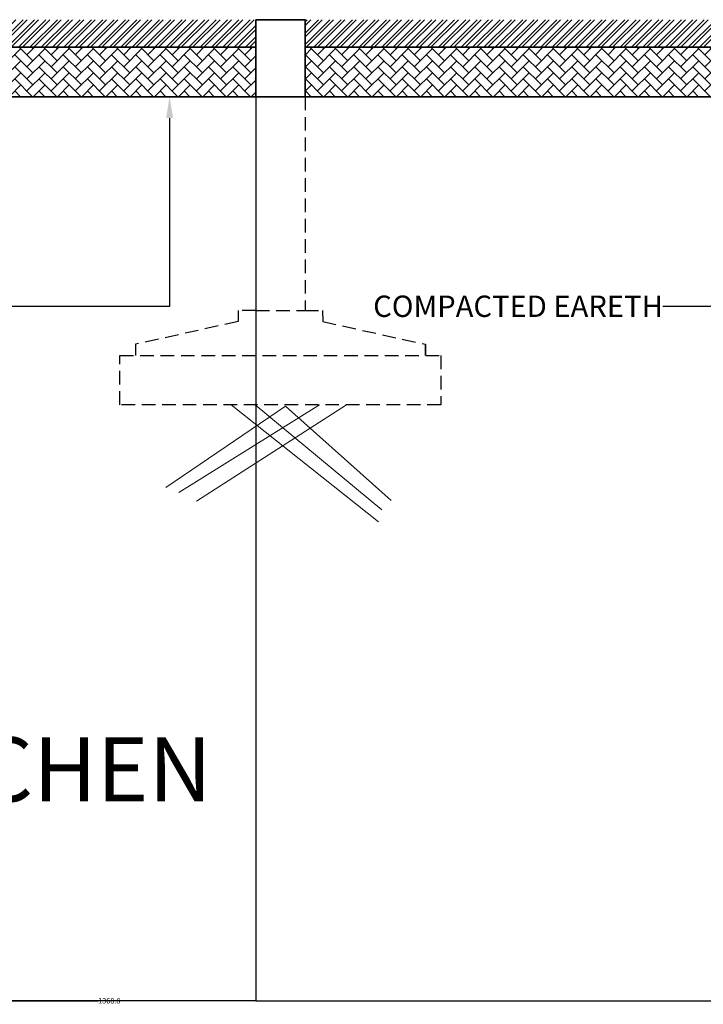
# Model space of a CAD drawing. Units: millimetres. Extents: x 1944 to 29915, y -10550 to 5909.
# Tile 18 of 24: x 19652 to 22846, y -10550 to -5946. Entities that reach past the tile are written whole.
import ezdxf
from ezdxf import colors
from ezdxf.entities.mleader import LeaderData, LeaderLine
from ezdxf.math import Vec2, Vec3

# ---------------------------------------------------------------- set-up
doc = ezdxf.new("R2010")
doc.units = ezdxf.units.MM
doc.header["$MEASUREMENT"] = 0
doc.linetypes.add('HIDDEN', pattern=[9.525, 6.35, -3.175])
for name, color, linetype, lineweight in [('A-ANNO-DIMS', 2, 'Continuous', 18), ('A-ANNO-TEXT', 7, 'Continuous', 25), ('A-FLOR-PATT', 252, 'Continuous', 13), ('A-SECT', 7, 'Continuous', 35), ('C-TOPO', 94, 'Continuous', 18), ('S-FNDN-HIDN', 1, 'HIDDEN', 25)]:
    doc.layers.add(name, color=color, linetype=linetype, lineweight=lineweight)
doc.styles.get("Standard").update_dxf_attribs({"font": 'arial.ttf'})
doc.dimstyles.get("Standard").update_dxf_attribs({"dimtxt": 25, "dimasz": 0.18, "dimexe": 0.18, "dimexo": 0.0625, "dimgap": 0.09, "dimtad": 0, "dimtih": 1, "dimtoh": 1, "dimdec": 0, "dimzin": 0, "dimdsep": 46, "dimtxsty": 'Standard', "dimcen": 0.09, "dimadec": 0, "dimazin": 0, "dimtfac": 1, "dimtdec": 0, "dimtofl": 0, "dimtmove": 0, "dimatfit": 3, "dimfxl": 1, "dimtolj": 1, "dimtzin": 0, "dimarcsym": 0})

# ---------------------------------------------------------------- blocks, each defined once
blk = doc.blocks.new('EARTH-COMPACT-SYMB')
for q in [(0, 60.9), (1053, 0)]:
    blk.add_line((559.8, 441.1), q)
blk = doc.blocks.new('*D88')
at = {"layer": 'A-ANNO-DIMS', "color": 0, "lineweight": -2, "transparency": 16777216}
for p, q in [((16747.8, -6305.8), (16747.8, -10533.3)), ((20755.4, -6305.8), (20755.4, -10533.3)), ((16748, -10533.1), (18713.7, -10533.1)), ((20755.3, -10533.1), (18789.6, -10533.1))]:
    blk.add_line(p, q, dxfattribs=at)
at = {"layer": 'A-ANNO-DIMS', "color": 0, "transparency": 16777216}
for points in [[(16748, -10533.1), (16748, -10533.1), (16747.8, -10533.1)], [(20755.3, -10533.1), (20755.3, -10533.1), (20755.4, -10533.1)]]:
    blk.add_solid(points, dxfattribs=at)
at = {"layer": 'Defpoints', "color": 0, "transparency": 16777216}
for p in [(16747.8, -6305.8), (20755.4, -6305.8), (20755.4, -10533.1)]:
    blk.add_point(p, dxfattribs=at)
at = {"layer": 'A-ANNO-DIMS', "color": 0, "transparency": 16777216, "insert": (18751.6, -10533.1), "char_height": 25, "attachment_point": 5}
blk.add_mtext('\\A1;4008', dxfattribs=at)
blk = doc.blocks.new('*D89')
at = {"layer": 'A-ANNO-DIMS', "color": 0, "lineweight": -2, "transparency": 16777216}
for p, q in [((20755.4, -6305.8), (20755.4, -10533.3)), ((25158, -6305.8), (25158, -10533.3)), ((20755.6, -10533.1), (22918.8, -10533.1)), ((25157.8, -10533.1), (22994.7, -10533.1))]:
    blk.add_line(p, q, dxfattribs=at)
at = {"layer": 'A-ANNO-DIMS', "color": 0, "transparency": 16777216}
for points in [[(20755.6, -10533.1), (20755.6, -10533.1), (20755.4, -10533.1)], [(25157.8, -10533.1), (25157.8, -10533.1), (25158, -10533.1)]]:
    blk.add_solid(points, dxfattribs=at)
at = {"layer": 'Defpoints', "color": 0, "transparency": 16777216}
for p in [(20755.4, -6305.8), (25158, -6305.8), (25158, -10533.1)]:
    blk.add_point(p, dxfattribs=at)
at = {"layer": 'A-ANNO-DIMS', "color": 0, "transparency": 16777216, "insert": (22956.7, -10533.1), "char_height": 25, "attachment_point": 5}
blk.add_mtext('\\A1;4403', dxfattribs=at)
blk = doc.blocks.new('*D98')
at = {"layer": 'A-ANNO-DIMS', "color": 0, "lineweight": -2, "transparency": 16777216}
for p, q in [((19386.6, -5945.8), (19386.6, -10533.3)), ((20755.4, -5945.8), (20755.4, -10533.3)), ((19386.8, -10533.1), (20020.2, -10533.1)), ((20755.3, -10533.1), (20121.9, -10533.1))]:
    blk.add_line(p, q, dxfattribs=at)
at = {"layer": 'A-ANNO-DIMS', "color": 0, "transparency": 16777216}
for points in [[(19386.8, -10533.1), (19386.8, -10533.1), (19386.6, -10533.1)], [(20755.3, -10533.1), (20755.3, -10533.1), (20755.4, -10533.1)]]:
    blk.add_solid(points, dxfattribs=at)
at = {"layer": 'Defpoints', "color": 0, "transparency": 16777216}
for p in [(19386.6, -5945.8), (20755.4, -5945.8), (20755.4, -10533.1)]:
    blk.add_point(p, dxfattribs=at)
at = {"layer": 'A-ANNO-DIMS', "color": 0, "transparency": 16777216, "insert": (20071, -10533.1), "char_height": 25, "attachment_point": 5}
blk.add_mtext('\\A1;1368.8', dxfattribs=at)

msp = doc.modelspace()

# ---------------------------------------------------------------- hatches: boundary and pattern name
at = {"layer": 'A-FLOR-PATT'}
h = msp.add_hatch(dxfattribs=at)
h.set_pattern_fill('ANSI32', color=256, scale=100)
h.paths.add_polyline_path([(16977.828, -5945.752), (16977.828, -6073.852), (20755.45, -6073.852), (20755.45, -5945.752)])
h = msp.add_hatch(dxfattribs=at)
h.set_pattern_fill('ANSI32', color=256, scale=100)
h.paths.add_polyline_path([(25159.297, -5945.752), (20985.45, -5945.752), (20985.45, -6073.852), (25159.297, -6073.852)])
h = msp.add_hatch(dxfattribs=at)
h.set_pattern_fill('AR-HBONE', color=256, scale=10)
h.paths.add_polyline_path([(20755.45, -6073.852), (16977.828, -6073.852), (16977.828, -6305.752), (20755.45, -6305.752)])
h = msp.add_hatch(dxfattribs=at)
h.set_pattern_fill('AR-HBONE', color=256, scale=10)
h.paths.add_polyline_path([(25159.297, -6073.852), (20985.45, -6073.852), (20985.45, -6305.752), (25159.297, -6305.752)])

# ---------------------------------------------------------------- linework, layer by layer
at = {"layer": 'A-SECT'}
for p, q in [((16977.828, -6073.852), (20755.45, -6073.852)), ((20985.45, -6073.852), (25159.297, -6073.852)), ((16977.828, -6305.752), (20755.45, -6305.752)), ((20985.45, -6305.752), (25159.297, -6305.752)), ((21548.074, -7463.338), (21548.074, -7516.218))]:
    msp.add_line(p, q, dxfattribs=at)
msp.add_lwpolyline([(20755.45, -5945.752), (20985.45, -5945.752), (20985.45, -6305.752), (20755.45, -6305.752)], close=True, dxfattribs=at)
at = {"layer": 'C-TOPO'}
for p, q in [((21053.683, -7746.218), (20395.385, -8155.847)), ((21178.637, -7746.218), (20479.196, -8196.963)), ((20640.723, -7746.218), (21329.497, -8292.9)), ((20751.963, -7746.218), (21344.736, -8238.079))]:
    msp.add_line(p, q, dxfattribs=at)
at = {"layer": 'S-FNDN-HIDN', "ltscale": 10}
for p, q in [((20755.45, -6305.752), (20755.45, -7305.752)), ((20985.45, -6305.752), (20985.45, -7305.752)), ((20673.421, -7304.748), (20672.778, -7357.264)), ((20755.45, -7305.752), (20673.421, -7304.748)), ((20755.45, -7305.752), (20985.45, -7305.752)), ((20985.45, -7305.752), (21067.479, -7304.748)), ((21067.479, -7304.748), (21068.121, -7357.264)), ((20672.778, -7357.264), (20192.826, -7463.338)), ((21068.121, -7357.264), (21548.074, -7463.338)), ((20192.826, -7463.338), (20192.826, -7516.218))]:
    msp.add_line(p, q, dxfattribs=at)
msp.add_lwpolyline([(20120.45, -7516.218), (21620.45, -7516.218), (21620.45, -7746.218), (20120.45, -7746.218)], close=True, dxfattribs=at)

# ---------------------------------------------------------------- block references
at = {"layer": 'C-TOPO'}
msp.add_blockref('EARTH-COMPACT-SYMB', (20334.431, -8193.917), dxfattribs=at)

# ---------------------------------------------------------------- texts
at = {"layer": 'A-ANNO-TEXT'}
msp.add_text('DETAILS OF  KITCHEN', height=300, dxfattribs=at).set_placement((16416.91, -9601.103))

# ---------------------------------------------------------------- dimensions: what is measured, and where the dimension line sits
at = {"layer": 'A-ANNO-DIMS'}
for base, p1, p2, override, picture, middle in [((20755.45, -10533.115), (19386.639, -5945.752), (20755.45, -5945.752), {"dimdec": 1, "dimlfac": 1, "dimrnd": 0, "dimzin": 0, "dimdsep": 46, "dimlunit": 2}, '*D98', (20071.044, -10533.115)), ((20755.45, -10533.115), (16747.828, -6305.752), (20755.45, -6305.752), {"dimdec": 0, "dimlfac": 1, "dimrnd": 0, "dimzin": 0, "dimdsep": 46, "dimlunit": 2}, '*D88', (18751.639, -10533.115)), ((25158.02, -10533.115), (20755.45, -6305.752), (25158.02, -6305.752), {"dimdec": 0, "dimlfac": 1, "dimrnd": 0, "dimzin": 0, "dimdsep": 46, "dimlunit": 2}, '*D89', (22956.735, -10533.115))]:
    dim = msp.add_linear_dim(base=base, p1=p1, p2=p2, dimstyle='Standard', override=override, dxfattribs=at)
    dim.commit()
    dim.dimension.update_dxf_attribs({"geometry": picture, "text_midpoint": middle})

# ---------------------------------------------------------------- leaders
at = {"layer": 'A-ANNO-TEXT'}
ml = msp.add_multileader_mtext('Standard', dxfattribs=at)
ml.set_content('COMPACTED EARETH ', color=256)
ml.set_leader_properties()
ml.build(insert=Vec2(0, 0))
ml.multileader.update_dxf_attribs({"dogleg_length": 568.936, "arrow_head_size": 100})
ctx = ml.context
ctx.base_point, ctx.char_height, ctx.arrow_head_size, ctx.landing_gap_size, ctx.plane_origin = Vec3(17154.841, -7286.495), 100, 100, 0.09, Vec3(19203.765, -7286.495)
ctx.text_align_type = 2
notes = []
notes.append((ctx, [(0, (1, 1, 0), (19203.765, -7286.495), (-1, 0), 568.936, [(0, [(20352.82, -6305.752), (20352.82, -7286.495)], 0, [])])]))
ctx.mtext.insert, ctx.mtext.alignment, ctx.mtext.flow_direction = Vec3(18634.74, -7235.642), 3, 5
ml = msp.add_multileader_mtext('Standard', dxfattribs=at)
ml.set_content('COMPACTED EARETH ', color=256)
ml.set_leader_properties()
ml.build(insert=Vec2(0, 0))
ml.multileader.update_dxf_attribs({"dogleg_length": 568.936, "arrow_head_size": 100})
ctx = ml.context
ctx.base_point, ctx.char_height, ctx.arrow_head_size, ctx.landing_gap_size, ctx.plane_origin = Vec3(21177.361, -7286.495), 100, 100, 0.09, Vec3(23226.285, -7286.495)
ctx.text_align_type = 2
notes.append((ctx, [(0, (1, 1, 0), (23226.285, -7286.495), (-1, 0), 568.936, [(0, [(24375.34, -6305.752), (24375.34, -7286.495)], 0, [])])]))
ctx.mtext.insert, ctx.mtext.alignment, ctx.mtext.flow_direction = Vec3(22657.26, -7235.642), 3, 5
for ctx, leaders in notes:
    for number, flags, end, landing, length, lines in leaders:
        leader = LeaderData()
        leader.index, (leader.has_last_leader_line, leader.has_dogleg_vector, leader.attachment_direction) = number, flags
        leader.last_leader_point, leader.dogleg_vector, leader.dogleg_length = Vec3(end), Vec3(landing), length
        for number, points, colour, breaks in lines:
            line = LeaderLine()
            line.index, line.vertices, line.color, line.breaks = number, Vec3.list(points), colors.encode_raw_color(colour), breaks
            leader.lines.append(line)
        ctx.leaders.append(leader)

doc.saveas('drawing.dxf')
